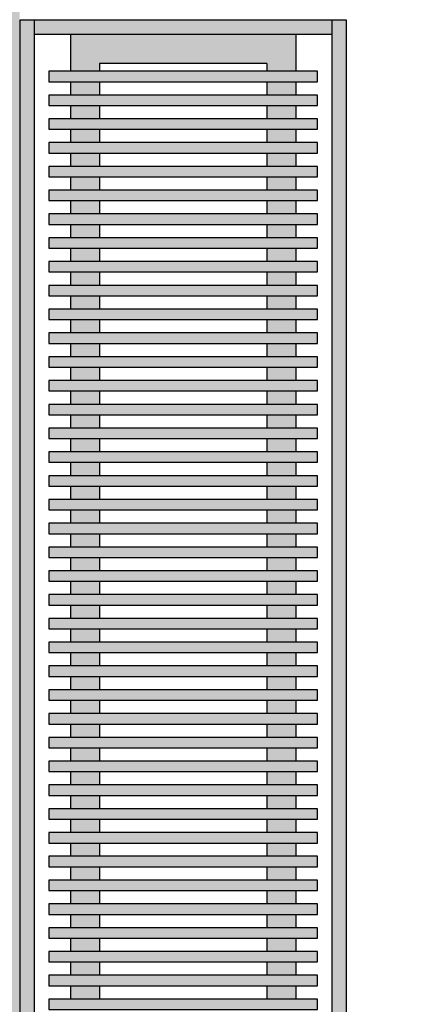
# Model space of a CAD drawing. Units: inches. Extents: x 3592 to 4861, y 1650 to 2243.
# Tile 20 of 30: x 4047 to 4068, y 2072 to 2125. Entities that reach past the tile are written whole.
import ezdxf

# ---------------------------------------------------------------- set-up
doc = ezdxf.new("R2010")
doc.units = ezdxf.units.IN
doc.layers.add('A-FURN', color=9, linetype='Continuous', lineweight=13)
doc.layers.add('estofado', color=7, linetype='Continuous', lineweight=25)
doc.layers.add('A-WALL-PATT', color=252, linetype='Continuous', lineweight=13, true_color=0x939598)
doc.layers.add('MOBIL', color=7, linetype='Continuous')

# ---------------------------------------------------------------- blocks, each defined once
blk = doc.blocks.new('Aparador Aido WV')
at = {"layer": 'MOBIL'}
h = blk.add_hatch(color=256, dxfattribs=at)
h.set_gradient(color1=(226, 228, 228), one_color=1, tint=1, name='CYLINDER')
h.paths.add_polyline_path([(0.9, -0.02), (0.9, 0), (-0.9, 0), (-0.9, -0.02)])
h = blk.add_hatch(color=256, dxfattribs=at)
h.set_gradient(color1=(226, 228, 228), one_color=1, tint=1)
h.paths.add_polyline_path([(-0.88, -0.02), (-0.9, -0.02), (-0.9, -0.43), (-0.88, -0.43)])
h = blk.add_hatch(color=256, dxfattribs=at)
h.set_gradient(color1=(106, 79, 62), color2=(55, 41, 32), one_color=1, tint=0.17)
h.paths.add_polyline_path([(-0.8151, -0.0402), (-0.8295, -0.0402), (-0.8295, -0.4098), (-0.8151, -0.4098)])
h = blk.add_hatch(color=256, dxfattribs=at)
h.set_gradient(color1=(106, 79, 62), color2=(55, 41, 32), one_color=1, tint=0.17)
h.paths.add_polyline_path([(-0.7967, -0.0402), (-0.7967, -0.4098), (-0.7823, -0.4098), (-0.7823, -0.0402)])
h = blk.add_hatch(color=256, dxfattribs=at)
h.set_gradient(color1=(106, 79, 62), color2=(55, 41, 32), one_color=1, tint=0.17)
h.paths.add_polyline_path([(-0.764, -0.0402), (-0.764, -0.4098), (-0.7496, -0.4098), (-0.7496, -0.0402)])
h = blk.add_hatch(color=256, dxfattribs=at)
h.set_gradient(color1=(106, 79, 62), color2=(55, 41, 32), one_color=1, tint=0.17)
h.paths.add_polyline_path([(-0.7312, -0.0402), (-0.7312, -0.4098), (-0.7168, -0.4098), (-0.7168, -0.0402)])
h = blk.add_hatch(color=256, dxfattribs=at)
h.set_gradient(color1=(106, 79, 62), color2=(55, 41, 32), one_color=1, tint=0.17)
h.paths.add_polyline_path([(-0.6985, -0.0402), (-0.6985, -0.4098), (-0.6841, -0.4098), (-0.6841, -0.0402)])
h = blk.add_hatch(color=256, dxfattribs=at)
h.set_gradient(color1=(106, 79, 62), color2=(55, 41, 32), one_color=1, tint=0.17)
h.paths.add_polyline_path([(-0.6657, -0.0402), (-0.6657, -0.4098), (-0.6513, -0.4098), (-0.6513, -0.0402)])
h = blk.add_hatch(color=256, dxfattribs=at)
h.set_gradient(color1=(106, 79, 62), color2=(55, 41, 32), one_color=1, tint=0.17)
h.paths.add_polyline_path([(-0.633, -0.0402), (-0.633, -0.4098), (-0.6186, -0.4098), (-0.6186, -0.0402)])
h = blk.add_hatch(color=256, dxfattribs=at)
h.set_gradient(color1=(106, 79, 62), color2=(55, 41, 32), one_color=1, tint=0.17)
h.paths.add_polyline_path([(-0.6002, -0.0402), (-0.6002, -0.4098), (-0.5858, -0.4098), (-0.5858, -0.0402)])
h = blk.add_hatch(color=256, dxfattribs=at)
h.set_gradient(color1=(106, 79, 62), color2=(55, 41, 32), one_color=1, tint=0.17)
h.paths.add_polyline_path([(-0.5675, -0.4098), (-0.5531, -0.4098), (-0.5531, -0.0402), (-0.5675, -0.0402)])
h = blk.add_hatch(color=256, dxfattribs=at)
h.set_gradient(color1=(106, 79, 62), color2=(55, 41, 32), one_color=1, tint=0.17)
h.paths.add_polyline_path([(-0.5347, -0.0402), (-0.5347, -0.4098), (-0.5203, -0.4098), (-0.5203, -0.0402)])
h = blk.add_hatch(color=256, dxfattribs=at)
h.set_gradient(color1=(106, 79, 62), color2=(55, 41, 32), one_color=1, tint=0.17)
h.paths.add_polyline_path([(-0.5019, -0.0402), (-0.5019, -0.4098), (-0.4876, -0.4098), (-0.4876, -0.0402)])
h = blk.add_hatch(color=256, dxfattribs=at)
h.set_gradient(color1=(106, 79, 62), color2=(55, 41, 32), one_color=1, tint=0.17)
h.paths.add_polyline_path([(-0.4692, -0.0402), (-0.4692, -0.4098), (-0.4548, -0.4098), (-0.4548, -0.0402)])
h = blk.add_hatch(color=256, dxfattribs=at)
h.set_gradient(color1=(106, 79, 62), color2=(55, 41, 32), one_color=1, tint=0.17)
h.paths.add_polyline_path([(-0.4364, -0.0402), (-0.4364, -0.4098), (-0.4221, -0.4098), (-0.4221, -0.0402)])
h = blk.add_hatch(color=256, dxfattribs=at)
h.set_gradient(color1=(106, 79, 62), color2=(55, 41, 32), one_color=1, tint=0.17)
h.paths.add_polyline_path([(-0.4037, -0.0402), (-0.4037, -0.4098), (-0.3893, -0.4098), (-0.3893, -0.0402)])
h = blk.add_hatch(color=256, dxfattribs=at)
h.set_gradient(color1=(106, 79, 62), color2=(55, 41, 32), one_color=1, tint=0.17)
h.paths.add_polyline_path([(-0.3709, -0.0402), (-0.3709, -0.4098), (-0.3566, -0.4098), (-0.3566, -0.0402)])
h = blk.add_hatch(color=256, dxfattribs=at)
h.set_gradient(color1=(106, 79, 62), color2=(55, 41, 32), one_color=1, tint=0.17)
h.paths.add_polyline_path([(-0.3382, -0.0402), (-0.3382, -0.4098), (-0.3238, -0.4098), (-0.3238, -0.0402)])
h = blk.add_hatch(color=256, dxfattribs=at)
h.set_gradient(color1=(106, 79, 62), color2=(55, 41, 32), one_color=1, tint=0.17)
h.paths.add_polyline_path([(-0.3054, -0.0402), (-0.3054, -0.4098), (-0.2911, -0.4098), (-0.2911, -0.0402)])
h = blk.add_hatch(color=256, dxfattribs=at)
h.set_gradient(color1=(106, 79, 62), color2=(55, 41, 32), one_color=1, tint=0.17)
h.paths.add_polyline_path([(-0.2727, -0.0402), (-0.2727, -0.4098), (-0.2583, -0.4098), (-0.2583, -0.0402)])
h = blk.add_hatch(color=256, dxfattribs=at)
h.set_gradient(color1=(106, 79, 62), color2=(55, 41, 32), one_color=1, tint=0.17)
h.paths.add_polyline_path([(-0.2399, -0.0402), (-0.2399, -0.4098), (-0.2256, -0.4098), (-0.2256, -0.0402)])
h = blk.add_hatch(color=256, dxfattribs=at)
h.set_gradient(color1=(106, 79, 62), color2=(55, 41, 32), one_color=1, tint=0.17)
h.paths.add_polyline_path([(-0.2072, -0.4098), (-0.1928, -0.4098), (-0.1928, -0.0402), (-0.2072, -0.0402)])
h = blk.add_hatch(color=256, dxfattribs=at)
h.set_gradient(color1=(106, 79, 62), color2=(55, 41, 32), one_color=1, tint=0.17)
h.paths.add_polyline_path([(-0.1744, -0.0402), (-0.1744, -0.4098), (-0.1601, -0.4098), (-0.1601, -0.0402)])
h = blk.add_hatch(color=256, dxfattribs=at)
h.set_gradient(color1=(106, 79, 62), color2=(55, 41, 32), one_color=1, tint=0.17)
h.paths.add_polyline_path([(-0.1417, -0.0402), (-0.1417, -0.4098), (-0.1273, -0.4098), (-0.1273, -0.0402)])
h = blk.add_hatch(color=256, dxfattribs=at)
h.set_gradient(color1=(106, 79, 62), color2=(55, 41, 32), one_color=1, tint=0.17)
h.paths.add_polyline_path([(-0.1089, -0.0402), (-0.1089, -0.4098), (-0.0946, -0.4098), (-0.0946, -0.0402)])
h = blk.add_hatch(color=256, dxfattribs=at)
h.set_gradient(color1=(106, 79, 62), color2=(55, 41, 32), one_color=1, tint=0.17)
h.paths.add_polyline_path([(-0.0762, -0.0402), (-0.0762, -0.4098), (-0.0618, -0.4098), (-0.0618, -0.0402)])
h = blk.add_hatch(color=256, dxfattribs=at)
h.set_gradient(color1=(106, 79, 62), color2=(55, 41, 32), one_color=1, tint=0.17)
h.paths.add_polyline_path([(-0.0434, -0.0402), (-0.0434, -0.4098), (-0.0291, -0.4098), (-0.0291, -0.0402)])
h = blk.add_hatch(color=256, dxfattribs=at)
h.set_gradient(color1=(106, 79, 62), color2=(55, 41, 32), one_color=1, tint=0.17)
h.paths.add_polyline_path([(-0.0107, -0.0402), (-0.0107, -0.4098), (0.0037, -0.4098), (0.0037, -0.0402)])
h = blk.add_hatch(color=256, dxfattribs=at)
h.set_gradient(color1=(106, 79, 62), color2=(55, 41, 32), one_color=1, tint=0.17)
h.paths.add_polyline_path([(0.0221, -0.0402), (0.0221, -0.4098), (0.0364, -0.4098), (0.0364, -0.0402)])
h = blk.add_hatch(color=256, dxfattribs=at)
h.set_gradient(color1=(106, 79, 62), color2=(55, 41, 32), one_color=1, tint=0.17)
h.paths.add_polyline_path([(0.0548, -0.0402), (0.0548, -0.4098), (0.0692, -0.4098), (0.0692, -0.0402)])
h = blk.add_hatch(color=256, dxfattribs=at)
h.set_gradient(color1=(106, 79, 62), color2=(55, 41, 32), one_color=1, tint=0.17)
h.paths.add_polyline_path([(0.1019, -0.0402), (0.0876, -0.0402), (0.0876, -0.4098), (0.1019, -0.4098)])
h = blk.add_hatch(color=256, dxfattribs=at)
h.set_gradient(color1=(106, 79, 62), color2=(55, 41, 32), one_color=1, tint=0.17)
h.paths.add_polyline_path([(0.1203, -0.0402), (0.1203, -0.4098), (0.1347, -0.4098), (0.1347, -0.0402)])
h = blk.add_hatch(color=256, dxfattribs=at)
h.set_gradient(color1=(106, 79, 62), color2=(55, 41, 32), one_color=1, tint=0.17)
h.paths.add_polyline_path([(0.1531, -0.0402), (0.1531, -0.4098), (0.1675, -0.4098), (0.1675, -0.0402)])
h = blk.add_hatch(color=256, dxfattribs=at)
h.set_gradient(color1=(106, 79, 62), color2=(55, 41, 32), one_color=1, tint=0.17)
h.paths.add_polyline_path([(0.1858, -0.0402), (0.1858, -0.4098), (0.2002, -0.4098), (0.2002, -0.0402)])
h = blk.add_hatch(color=256, dxfattribs=at)
h.set_gradient(color1=(106, 79, 62), color2=(55, 41, 32), one_color=1, tint=0.17)
h.paths.add_polyline_path([(0.2186, -0.0402), (0.2186, -0.4098), (0.233, -0.4098), (0.233, -0.0402)])
h = blk.add_hatch(color=256, dxfattribs=at)
h.set_gradient(color1=(106, 79, 62), color2=(55, 41, 32), one_color=1, tint=0.17)
h.paths.add_polyline_path([(0.2513, -0.0402), (0.2513, -0.4098), (0.2657, -0.4098), (0.2657, -0.0402)])
h = blk.add_hatch(color=256, dxfattribs=at)
h.set_gradient(color1=(106, 79, 62), color2=(55, 41, 32), one_color=1, tint=0.17)
h.paths.add_polyline_path([(0.2841, -0.0402), (0.2841, -0.4098), (0.2985, -0.4098), (0.2985, -0.0402)])
h = blk.add_hatch(color=256, dxfattribs=at)
h.set_gradient(color1=(106, 79, 62), color2=(55, 41, 32), one_color=1, tint=0.17)
h.paths.add_polyline_path([(0.3168, -0.0402), (0.3168, -0.4098), (0.3312, -0.4098), (0.3312, -0.0402)])
h = blk.add_hatch(color=256, dxfattribs=at)
h.set_gradient(color1=(106, 79, 62), color2=(55, 41, 32), one_color=1, tint=0.17)
h.paths.add_polyline_path([(0.3496, -0.0402), (0.3496, -0.4098), (0.364, -0.4098), (0.364, -0.0402)])
h = blk.add_hatch(color=256, dxfattribs=at)
h.set_gradient(color1=(106, 79, 62), color2=(55, 41, 32), one_color=1, tint=0.17)
h.paths.add_polyline_path([(0.3823, -0.0402), (0.3823, -0.4098), (0.3967, -0.4098), (0.3967, -0.0402)])
h = blk.add_hatch(color=256, dxfattribs=at)
h.set_gradient(color1=(106, 79, 62), color2=(55, 41, 32), one_color=1, tint=0.17)
h.paths.add_polyline_path([(0.4151, -0.4098), (0.4295, -0.4098), (0.4295, -0.0402), (0.4151, -0.0402)])
h = blk.add_hatch(color=256, dxfattribs=at)
h.set_gradient(color1=(106, 79, 62), color2=(55, 41, 32), one_color=1, tint=0.17)
h.paths.add_polyline_path([(0.4479, -0.0402), (0.4479, -0.4098), (0.4622, -0.4098), (0.4622, -0.0402)])
h = blk.add_hatch(color=256, dxfattribs=at)
h.set_gradient(color1=(106, 79, 62), color2=(157, 117, 92), one_color=1, tint=0.49)
h.paths.add_polyline_path([(-0.84, -0.11), (-0.8295, -0.11), (-0.8295, -0.07), (-0.88, -0.07), (-0.88, -0.38), (-0.8295, -0.38), (-0.8295, -0.34), (-0.84, -0.34)])
h = blk.add_hatch(color=256, dxfattribs=at)
h.set_gradient(color1=(106, 79, 62), color2=(157, 117, 92), one_color=1, tint=0.49)
h.paths.add_polyline_path([(-0.7967, -0.07), (-0.8151, -0.07), (-0.8151, -0.11), (-0.7967, -0.11)])
h = blk.add_hatch(color=256, dxfattribs=at)
h.set_gradient(color1=(106, 79, 62), color2=(157, 117, 92), one_color=1, tint=0.49)
h.paths.add_polyline_path([(-0.764, -0.07), (-0.7823, -0.07), (-0.7823, -0.11), (-0.764, -0.11)])
h = blk.add_hatch(color=256, dxfattribs=at)
h.set_gradient(color1=(106, 79, 62), color2=(157, 117, 92), one_color=1, tint=0.49)
h.paths.add_polyline_path([(-0.7312, -0.07), (-0.7496, -0.07), (-0.7496, -0.11), (-0.7312, -0.11)])
h = blk.add_hatch(color=256, dxfattribs=at)
h.set_gradient(color1=(106, 79, 62), color2=(157, 117, 92), one_color=1, tint=0.49)
h.paths.add_polyline_path([(-0.6985, -0.07), (-0.7168, -0.07), (-0.7168, -0.11), (-0.6985, -0.11)])
h = blk.add_hatch(color=256, dxfattribs=at)
h.set_gradient(color1=(106, 79, 62), color2=(157, 117, 92), one_color=1, tint=0.49)
h.paths.add_polyline_path([(-0.6657, -0.07), (-0.6841, -0.07), (-0.6841, -0.11), (-0.6657, -0.11)])
h = blk.add_hatch(color=256, dxfattribs=at)
h.set_gradient(color1=(106, 79, 62), color2=(157, 117, 92), one_color=1, tint=0.49)
h.paths.add_polyline_path([(-0.633, -0.07), (-0.6513, -0.07), (-0.6513, -0.11), (-0.633, -0.11)])
h = blk.add_hatch(color=256, dxfattribs=at)
h.set_gradient(color1=(106, 79, 62), color2=(157, 117, 92), one_color=1, tint=0.49)
h.paths.add_polyline_path([(-0.6002, -0.07), (-0.6186, -0.07), (-0.6186, -0.11), (-0.6002, -0.11)])
h = blk.add_hatch(color=256, dxfattribs=at)
h.set_gradient(color1=(106, 79, 62), color2=(157, 117, 92), one_color=1, tint=0.49)
h.paths.add_polyline_path([(-0.5675, -0.07), (-0.5858, -0.07), (-0.5858, -0.11), (-0.5675, -0.11)])
h = blk.add_hatch(color=256, dxfattribs=at)
h.set_gradient(color1=(106, 79, 62), color2=(157, 117, 92), one_color=1, tint=0.49)
h.paths.add_polyline_path([(-0.5347, -0.07), (-0.5531, -0.07), (-0.5531, -0.11), (-0.5347, -0.11)])
h = blk.add_hatch(color=256, dxfattribs=at)
h.set_gradient(color1=(106, 79, 62), color2=(157, 117, 92), one_color=1, tint=0.49)
h.paths.add_polyline_path([(-0.5019, -0.07), (-0.5203, -0.07), (-0.5203, -0.11), (-0.5019, -0.11)])
h = blk.add_hatch(color=256, dxfattribs=at)
h.set_gradient(color1=(106, 79, 62), color2=(157, 117, 92), one_color=1, tint=0.49)
h.paths.add_polyline_path([(-0.4692, -0.07), (-0.4876, -0.07), (-0.4876, -0.11), (-0.4692, -0.11)])
h = blk.add_hatch(color=256, dxfattribs=at)
h.set_gradient(color1=(106, 79, 62), color2=(157, 117, 92), one_color=1, tint=0.49)
h.paths.add_polyline_path([(-0.4364, -0.07), (-0.4548, -0.07), (-0.4548, -0.11), (-0.4364, -0.11)])
h = blk.add_hatch(color=256, dxfattribs=at)
h.set_gradient(color1=(106, 79, 62), color2=(157, 117, 92), one_color=1, tint=0.49)
h.paths.add_polyline_path([(-0.4037, -0.07), (-0.4221, -0.07), (-0.4221, -0.11), (-0.4037, -0.11)])
h = blk.add_hatch(color=256, dxfattribs=at)
h.set_gradient(color1=(106, 79, 62), color2=(157, 117, 92), one_color=1, tint=0.49)
h.paths.add_polyline_path([(-0.3709, -0.07), (-0.3893, -0.07), (-0.3893, -0.11), (-0.3709, -0.11)])
h = blk.add_hatch(color=256, dxfattribs=at)
h.set_gradient(color1=(106, 79, 62), color2=(157, 117, 92), one_color=1, tint=0.49)
h.paths.add_polyline_path([(-0.3382, -0.07), (-0.3566, -0.07), (-0.3566, -0.11), (-0.3382, -0.11)])
h = blk.add_hatch(color=256, dxfattribs=at)
h.set_gradient(color1=(106, 79, 62), color2=(157, 117, 92), one_color=1, tint=0.49)
h.paths.add_polyline_path([(-0.3054, -0.07), (-0.3238, -0.07), (-0.3238, -0.11), (-0.3054, -0.11)])
h = blk.add_hatch(color=256, dxfattribs=at)
h.set_gradient(color1=(106, 79, 62), color2=(157, 117, 92), one_color=1, tint=0.49)
h.paths.add_polyline_path([(-0.2727, -0.07), (-0.2911, -0.07), (-0.2911, -0.11), (-0.2727, -0.11)])
h = blk.add_hatch(color=256, dxfattribs=at)
h.set_gradient(color1=(106, 79, 62), color2=(157, 117, 92), one_color=1, tint=0.49)
h.paths.add_polyline_path([(-0.2399, -0.07), (-0.2583, -0.07), (-0.2583, -0.11), (-0.2399, -0.11)])
h = blk.add_hatch(color=256, dxfattribs=at)
h.set_gradient(color1=(106, 79, 62), color2=(157, 117, 92), one_color=1, tint=0.49)
h.paths.add_polyline_path([(-0.2072, -0.07), (-0.2256, -0.07), (-0.2256, -0.11), (-0.2072, -0.11)])
h = blk.add_hatch(color=256, dxfattribs=at)
h.set_gradient(color1=(106, 79, 62), color2=(157, 117, 92), one_color=1, tint=0.49)
h.paths.add_polyline_path([(-0.1744, -0.07), (-0.1928, -0.07), (-0.1928, -0.11), (-0.1744, -0.11)])
h = blk.add_hatch(color=256, dxfattribs=at)
h.set_gradient(color1=(106, 79, 62), color2=(157, 117, 92), one_color=1, tint=0.49)
h.paths.add_polyline_path([(-0.1417, -0.07), (-0.1601, -0.07), (-0.1601, -0.11), (-0.1417, -0.11)])
h = blk.add_hatch(color=256, dxfattribs=at)
h.set_gradient(color1=(106, 79, 62), color2=(157, 117, 92), one_color=1, tint=0.49)
h.paths.add_polyline_path([(-0.1089, -0.07), (-0.1273, -0.07), (-0.1273, -0.11), (-0.1089, -0.11)])
h = blk.add_hatch(color=256, dxfattribs=at)
h.set_gradient(color1=(106, 79, 62), color2=(157, 117, 92), one_color=1, tint=0.49)
h.paths.add_polyline_path([(-0.0762, -0.07), (-0.0946, -0.07), (-0.0946, -0.11), (-0.0762, -0.11)])
h = blk.add_hatch(color=256, dxfattribs=at)
h.set_gradient(color1=(106, 79, 62), color2=(157, 117, 92), one_color=1, tint=0.49)
h.paths.add_polyline_path([(-0.0434, -0.07), (-0.0618, -0.07), (-0.0618, -0.11), (-0.0434, -0.11)])
h = blk.add_hatch(color=256, dxfattribs=at)
h.set_gradient(color1=(106, 79, 62), color2=(157, 117, 92), one_color=1, tint=0.49)
h.paths.add_polyline_path([(-0.0107, -0.07), (-0.0291, -0.07), (-0.0291, -0.11), (-0.0107, -0.11)])
h = blk.add_hatch(color=256, dxfattribs=at)
h.set_gradient(color1=(106, 79, 62), color2=(157, 117, 92), one_color=1, tint=0.49)
h.paths.add_polyline_path([(0.0221, -0.07), (0.0037, -0.07), (0.0037, -0.11), (0.0221, -0.11)])
h = blk.add_hatch(color=256, dxfattribs=at)
h.set_gradient(color1=(106, 79, 62), color2=(157, 117, 92), one_color=1, tint=0.49)
h.paths.add_polyline_path([(0.0548, -0.07), (0.0364, -0.07), (0.0364, -0.11), (0.0548, -0.11)])
h = blk.add_hatch(color=256, dxfattribs=at)
h.set_gradient(color1=(106, 79, 62), color2=(157, 117, 92), one_color=1, tint=0.49)
h.paths.add_polyline_path([(0.0876, -0.07), (0.0692, -0.07), (0.0692, -0.11), (0.0876, -0.11)])
h = blk.add_hatch(color=256, dxfattribs=at)
h.set_gradient(color1=(106, 79, 62), color2=(157, 117, 92), one_color=1, tint=0.49)
h.paths.add_polyline_path([(0.1203, -0.07), (0.1019, -0.07), (0.1019, -0.11), (0.1203, -0.11)])
h = blk.add_hatch(color=256, dxfattribs=at)
h.set_gradient(color1=(106, 79, 62), color2=(157, 117, 92), one_color=1, tint=0.49)
h.paths.add_polyline_path([(0.1531, -0.07), (0.1347, -0.07), (0.1347, -0.11), (0.1531, -0.11)])
h = blk.add_hatch(color=256, dxfattribs=at)
h.set_gradient(color1=(106, 79, 62), color2=(157, 117, 92), one_color=1, tint=0.49)
h.paths.add_polyline_path([(0.1858, -0.07), (0.1675, -0.07), (0.1675, -0.11), (0.1858, -0.11)])
h = blk.add_hatch(color=256, dxfattribs=at)
h.set_gradient(color1=(106, 79, 62), color2=(157, 117, 92), one_color=1, tint=0.49)
h.paths.add_polyline_path([(0.2186, -0.07), (0.2002, -0.07), (0.2002, -0.11), (0.2186, -0.11)])
h = blk.add_hatch(color=256, dxfattribs=at)
h.set_gradient(color1=(106, 79, 62), color2=(157, 117, 92), one_color=1, tint=0.49)
h.paths.add_polyline_path([(0.2513, -0.07), (0.233, -0.07), (0.233, -0.11), (0.2513, -0.11)])
h = blk.add_hatch(color=256, dxfattribs=at)
h.set_gradient(color1=(106, 79, 62), color2=(157, 117, 92), one_color=1, tint=0.49)
h.paths.add_polyline_path([(0.2841, -0.07), (0.2657, -0.07), (0.2657, -0.11), (0.2841, -0.11)])
h = blk.add_hatch(color=256, dxfattribs=at)
h.set_gradient(color1=(106, 79, 62), color2=(157, 117, 92), one_color=1, tint=0.49)
h.paths.add_polyline_path([(0.3168, -0.07), (0.2985, -0.07), (0.2985, -0.11), (0.3168, -0.11)])
h = blk.add_hatch(color=256, dxfattribs=at)
h.set_gradient(color1=(106, 79, 62), color2=(157, 117, 92), one_color=1, tint=0.49)
h.paths.add_polyline_path([(0.3496, -0.07), (0.3312, -0.07), (0.3312, -0.11), (0.3496, -0.11)])
h = blk.add_hatch(color=256, dxfattribs=at)
h.set_gradient(color1=(106, 79, 62), color2=(157, 117, 92), one_color=1, tint=0.49)
h.paths.add_polyline_path([(0.3823, -0.07), (0.364, -0.07), (0.364, -0.11), (0.3823, -0.11)])
h = blk.add_hatch(color=256, dxfattribs=at)
h.set_gradient(color1=(106, 79, 62), color2=(157, 117, 92), one_color=1, tint=0.49)
h.paths.add_polyline_path([(0.4151, -0.07), (0.3967, -0.07), (0.3967, -0.11), (0.4151, -0.11)])
h = blk.add_hatch(color=256, dxfattribs=at)
h.set_gradient(color1=(106, 79, 62), color2=(157, 117, 92), one_color=1, tint=0.49)
h.paths.add_polyline_path([(0.4479, -0.07), (0.4295, -0.07), (0.4295, -0.11), (0.4479, -0.11)])
h = blk.add_hatch(color=256, dxfattribs=at)
h.set_gradient(color1=(106, 79, 62), color2=(157, 117, 92), one_color=1, tint=0.49)
h.paths.add_polyline_path([(-0.7967, -0.34), (-0.8151, -0.34), (-0.8151, -0.38), (-0.7967, -0.38)])
h = blk.add_hatch(color=256, dxfattribs=at)
h.set_gradient(color1=(106, 79, 62), color2=(157, 117, 92), one_color=1, tint=0.49)
h.paths.add_polyline_path([(-0.764, -0.34), (-0.7823, -0.34), (-0.7823, -0.38), (-0.764, -0.38)])
h = blk.add_hatch(color=256, dxfattribs=at)
h.set_gradient(color1=(106, 79, 62), color2=(157, 117, 92), one_color=1, tint=0.49)
h.paths.add_polyline_path([(-0.7312, -0.34), (-0.7496, -0.34), (-0.7496, -0.38), (-0.7312, -0.38)])
h = blk.add_hatch(color=256, dxfattribs=at)
h.set_gradient(color1=(106, 79, 62), color2=(157, 117, 92), one_color=1, tint=0.49)
h.paths.add_polyline_path([(-0.6985, -0.34), (-0.7168, -0.34), (-0.7168, -0.38), (-0.6985, -0.38)])
h = blk.add_hatch(color=256, dxfattribs=at)
h.set_gradient(color1=(106, 79, 62), color2=(157, 117, 92), one_color=1, tint=0.49)
h.paths.add_polyline_path([(-0.6657, -0.34), (-0.6841, -0.34), (-0.6841, -0.38), (-0.6657, -0.38)])
h = blk.add_hatch(color=256, dxfattribs=at)
h.set_gradient(color1=(106, 79, 62), color2=(157, 117, 92), one_color=1, tint=0.49)
h.paths.add_polyline_path([(-0.633, -0.34), (-0.6513, -0.34), (-0.6513, -0.38), (-0.633, -0.38)])
h = blk.add_hatch(color=256, dxfattribs=at)
h.set_gradient(color1=(106, 79, 62), color2=(157, 117, 92), one_color=1, tint=0.49)
h.paths.add_polyline_path([(-0.6002, -0.34), (-0.6186, -0.34), (-0.6186, -0.38), (-0.6002, -0.38)])
h = blk.add_hatch(color=256, dxfattribs=at)
h.set_gradient(color1=(106, 79, 62), color2=(157, 117, 92), one_color=1, tint=0.49)
h.paths.add_polyline_path([(-0.5675, -0.34), (-0.5858, -0.34), (-0.5858, -0.38), (-0.5675, -0.38)])
h = blk.add_hatch(color=256, dxfattribs=at)
h.set_gradient(color1=(106, 79, 62), color2=(157, 117, 92), one_color=1, tint=0.49)
h.paths.add_polyline_path([(-0.5347, -0.34), (-0.5531, -0.34), (-0.5531, -0.38), (-0.5347, -0.38)])
h = blk.add_hatch(color=256, dxfattribs=at)
h.set_gradient(color1=(106, 79, 62), color2=(157, 117, 92), one_color=1, tint=0.49)
h.paths.add_polyline_path([(-0.5019, -0.34), (-0.5203, -0.34), (-0.5203, -0.38), (-0.5019, -0.38)])
h = blk.add_hatch(color=256, dxfattribs=at)
h.set_gradient(color1=(106, 79, 62), color2=(157, 117, 92), one_color=1, tint=0.49)
h.paths.add_polyline_path([(-0.4692, -0.34), (-0.4876, -0.34), (-0.4876, -0.38), (-0.4692, -0.38)])
h = blk.add_hatch(color=256, dxfattribs=at)
h.set_gradient(color1=(106, 79, 62), color2=(157, 117, 92), one_color=1, tint=0.49)
h.paths.add_polyline_path([(-0.4364, -0.34), (-0.4548, -0.34), (-0.4548, -0.38), (-0.4364, -0.38)])
h = blk.add_hatch(color=256, dxfattribs=at)
h.set_gradient(color1=(106, 79, 62), color2=(157, 117, 92), one_color=1, tint=0.49)
h.paths.add_polyline_path([(-0.4037, -0.34), (-0.4221, -0.34), (-0.4221, -0.38), (-0.4037, -0.38)])
h = blk.add_hatch(color=256, dxfattribs=at)
h.set_gradient(color1=(106, 79, 62), color2=(157, 117, 92), one_color=1, tint=0.49)
h.paths.add_polyline_path([(-0.3709, -0.34), (-0.3893, -0.34), (-0.3893, -0.38), (-0.3709, -0.38)])
h = blk.add_hatch(color=256, dxfattribs=at)
h.set_gradient(color1=(106, 79, 62), color2=(157, 117, 92), one_color=1, tint=0.49)
h.paths.add_polyline_path([(-0.3382, -0.34), (-0.3566, -0.34), (-0.3566, -0.38), (-0.3382, -0.38)])
h = blk.add_hatch(color=256, dxfattribs=at)
h.set_gradient(color1=(106, 79, 62), color2=(157, 117, 92), one_color=1, tint=0.49)
h.paths.add_polyline_path([(-0.3054, -0.34), (-0.3238, -0.34), (-0.3238, -0.38), (-0.3054, -0.38)])
h = blk.add_hatch(color=256, dxfattribs=at)
h.set_gradient(color1=(106, 79, 62), color2=(157, 117, 92), one_color=1, tint=0.49)
h.paths.add_polyline_path([(-0.2727, -0.34), (-0.2911, -0.34), (-0.2911, -0.38), (-0.2727, -0.38)])
h = blk.add_hatch(color=256, dxfattribs=at)
h.set_gradient(color1=(106, 79, 62), color2=(157, 117, 92), one_color=1, tint=0.49)
h.paths.add_polyline_path([(-0.2399, -0.34), (-0.2583, -0.34), (-0.2583, -0.38), (-0.2399, -0.38)])
h = blk.add_hatch(color=256, dxfattribs=at)
h.set_gradient(color1=(106, 79, 62), color2=(157, 117, 92), one_color=1, tint=0.49)
h.paths.add_polyline_path([(-0.2072, -0.34), (-0.2256, -0.34), (-0.2256, -0.38), (-0.2072, -0.38)])
h = blk.add_hatch(color=256, dxfattribs=at)
h.set_gradient(color1=(106, 79, 62), color2=(157, 117, 92), one_color=1, tint=0.49)
h.paths.add_polyline_path([(-0.1744, -0.34), (-0.1928, -0.34), (-0.1928, -0.38), (-0.1744, -0.38)])
h = blk.add_hatch(color=256, dxfattribs=at)
h.set_gradient(color1=(106, 79, 62), color2=(157, 117, 92), one_color=1, tint=0.49)
h.paths.add_polyline_path([(-0.1417, -0.34), (-0.1601, -0.34), (-0.1601, -0.38), (-0.1417, -0.38)])
h = blk.add_hatch(color=256, dxfattribs=at)
h.set_gradient(color1=(106, 79, 62), color2=(157, 117, 92), one_color=1, tint=0.49)
h.paths.add_polyline_path([(-0.1089, -0.34), (-0.1273, -0.34), (-0.1273, -0.38), (-0.1089, -0.38)])
h = blk.add_hatch(color=256, dxfattribs=at)
h.set_gradient(color1=(106, 79, 62), color2=(157, 117, 92), one_color=1, tint=0.49)
h.paths.add_polyline_path([(-0.0762, -0.34), (-0.0946, -0.34), (-0.0946, -0.38), (-0.0762, -0.38)])
h = blk.add_hatch(color=256, dxfattribs=at)
h.set_gradient(color1=(106, 79, 62), color2=(157, 117, 92), one_color=1, tint=0.49)
h.paths.add_polyline_path([(-0.0434, -0.34), (-0.0618, -0.34), (-0.0618, -0.38), (-0.0434, -0.38)])
h = blk.add_hatch(color=256, dxfattribs=at)
h.set_gradient(color1=(106, 79, 62), color2=(157, 117, 92), one_color=1, tint=0.49)
h.paths.add_polyline_path([(-0.0107, -0.34), (-0.0291, -0.34), (-0.0291, -0.38), (-0.0107, -0.38)])
h = blk.add_hatch(color=256, dxfattribs=at)
h.set_gradient(color1=(106, 79, 62), color2=(157, 117, 92), one_color=1, tint=0.49)
h.paths.add_polyline_path([(0.0221, -0.34), (0.0037, -0.34), (0.0037, -0.38), (0.0221, -0.38)])
h = blk.add_hatch(color=256, dxfattribs=at)
h.set_gradient(color1=(106, 79, 62), color2=(157, 117, 92), one_color=1, tint=0.49)
h.paths.add_polyline_path([(0.0548, -0.34), (0.0364, -0.34), (0.0364, -0.38), (0.0548, -0.38)])
h = blk.add_hatch(color=256, dxfattribs=at)
h.set_gradient(color1=(106, 79, 62), color2=(157, 117, 92), one_color=1, tint=0.49)
h.paths.add_polyline_path([(0.0876, -0.34), (0.0692, -0.34), (0.0692, -0.38), (0.0876, -0.38)])
h = blk.add_hatch(color=256, dxfattribs=at)
h.set_gradient(color1=(106, 79, 62), color2=(157, 117, 92), one_color=1, tint=0.49)
h.paths.add_polyline_path([(0.1203, -0.34), (0.1019, -0.34), (0.1019, -0.38), (0.1203, -0.38)])
h = blk.add_hatch(color=256, dxfattribs=at)
h.set_gradient(color1=(106, 79, 62), color2=(157, 117, 92), one_color=1, tint=0.49)
h.paths.add_polyline_path([(0.1531, -0.34), (0.1347, -0.34), (0.1347, -0.38), (0.1531, -0.38)])
h = blk.add_hatch(color=256, dxfattribs=at)
h.set_gradient(color1=(106, 79, 62), color2=(157, 117, 92), one_color=1, tint=0.49)
h.paths.add_polyline_path([(0.1858, -0.34), (0.1675, -0.34), (0.1675, -0.38), (0.1858, -0.38)])
h = blk.add_hatch(color=256, dxfattribs=at)
h.set_gradient(color1=(106, 79, 62), color2=(157, 117, 92), one_color=1, tint=0.49)
h.paths.add_polyline_path([(0.2186, -0.34), (0.2002, -0.34), (0.2002, -0.38), (0.2186, -0.38)])
h = blk.add_hatch(color=256, dxfattribs=at)
h.set_gradient(color1=(106, 79, 62), color2=(157, 117, 92), one_color=1, tint=0.49)
h.paths.add_polyline_path([(0.2513, -0.34), (0.233, -0.34), (0.233, -0.38), (0.2513, -0.38)])
h = blk.add_hatch(color=256, dxfattribs=at)
h.set_gradient(color1=(106, 79, 62), color2=(157, 117, 92), one_color=1, tint=0.49)
h.paths.add_polyline_path([(0.2841, -0.34), (0.2657, -0.34), (0.2657, -0.38), (0.2841, -0.38)])
h = blk.add_hatch(color=256, dxfattribs=at)
h.set_gradient(color1=(106, 79, 62), color2=(157, 117, 92), one_color=1, tint=0.49)
h.paths.add_polyline_path([(0.3168, -0.34), (0.2985, -0.34), (0.2985, -0.38), (0.3168, -0.38)])
h = blk.add_hatch(color=256, dxfattribs=at)
h.set_gradient(color1=(106, 79, 62), color2=(157, 117, 92), one_color=1, tint=0.49)
h.paths.add_polyline_path([(0.3496, -0.34), (0.3312, -0.34), (0.3312, -0.38), (0.3496, -0.38)])
h = blk.add_hatch(color=256, dxfattribs=at)
h.set_gradient(color1=(106, 79, 62), color2=(157, 117, 92), one_color=1, tint=0.49)
h.paths.add_polyline_path([(0.3823, -0.34), (0.364, -0.34), (0.364, -0.38), (0.3823, -0.38)])
h = blk.add_hatch(color=256, dxfattribs=at)
h.set_gradient(color1=(106, 79, 62), color2=(157, 117, 92), one_color=1, tint=0.49)
h.paths.add_polyline_path([(0.4151, -0.34), (0.3967, -0.34), (0.3967, -0.38), (0.4151, -0.38)])
h = blk.add_hatch(color=256, dxfattribs=at)
h.set_gradient(color1=(106, 79, 62), color2=(157, 117, 92), one_color=1, tint=0.49)
h.paths.add_polyline_path([(0.4479, -0.34), (0.4295, -0.34), (0.4295, -0.38), (0.4479, -0.38)])
h = blk.add_hatch(color=256, dxfattribs=at)
h.set_gradient(color1=(226, 228, 228), one_color=1, tint=1, name='CYLINDER')
h.paths.add_polyline_path([(0.9, -0.45), (0.9, -0.43), (-0.9, -0.43), (-0.9, -0.45)])
at = {"layer": 'estofado', "ltscale": 0.5}
for p, q in [((-0.88, -0.07), (-0.8295, -0.07)), ((-0.8151, -0.07), (-0.7967, -0.07)), ((-0.7823, -0.07), (-0.764, -0.07)), ((-0.7496, -0.07), (-0.7312, -0.07)), ((-0.7168, -0.07), (-0.6985, -0.07)), ((-0.6841, -0.07), (-0.6657, -0.07)), ((-0.6513, -0.07), (-0.633, -0.07)), ((-0.6186, -0.07), (-0.6002, -0.07)), ((-0.5858, -0.07), (-0.5675, -0.07)), ((-0.5531, -0.07), (-0.5347, -0.07)), ((-0.5203, -0.07), (-0.5019, -0.07)), ((-0.4876, -0.07), (-0.4692, -0.07)), ((-0.4548, -0.07), (-0.4364, -0.07)), ((-0.4221, -0.07), (-0.4037, -0.07)), ((-0.3893, -0.07), (-0.3709, -0.07)), ((-0.3566, -0.07), (-0.3382, -0.07)), ((-0.3238, -0.07), (-0.3054, -0.07)), ((-0.2911, -0.07), (-0.2727, -0.07)), ((-0.2583, -0.07), (-0.2399, -0.07)), ((-0.2256, -0.07), (-0.2072, -0.07)), ((-0.1928, -0.07), (-0.1744, -0.07)), ((-0.1601, -0.07), (-0.1417, -0.07)), ((-0.1273, -0.07), (-0.1089, -0.07)), ((-0.0946, -0.07), (-0.0762, -0.07)), ((-0.0618, -0.07), (-0.0434, -0.07)), ((-0.0291, -0.07), (-0.0107, -0.07)), ((0.0037, -0.07), (0.0221, -0.07)), ((0.0364, -0.07), (0.0548, -0.07)), ((0.0692, -0.07), (0.0876, -0.07)), ((0.1019, -0.07), (0.1203, -0.07)), ((0.1347, -0.07), (0.1531, -0.07)), ((0.1675, -0.07), (0.1858, -0.07)), ((0.2002, -0.07), (0.2186, -0.07)), ((0.233, -0.07), (0.2513, -0.07)), ((0.2657, -0.07), (0.2841, -0.07)), ((0.2985, -0.07), (0.3168, -0.07)), ((0.3312, -0.07), (0.3496, -0.07)), ((0.364, -0.07), (0.3823, -0.07)), ((0.3967, -0.07), (0.4151, -0.07)), ((0.4295, -0.07), (0.4479, -0.07)), ((-0.84, -0.11), (-0.84, -0.34)), ((-0.84, -0.11), (-0.8295, -0.11)), ((-0.8151, -0.11), (-0.7967, -0.11)), ((-0.7823, -0.11), (-0.764, -0.11)), ((-0.7496, -0.11), (-0.7312, -0.11)), ((-0.7168, -0.11), (-0.6985, -0.11)), ((-0.6841, -0.11), (-0.6657, -0.11)), ((-0.6513, -0.11), (-0.633, -0.11)), ((-0.6186, -0.11), (-0.6002, -0.11)), ((-0.5858, -0.11), (-0.5675, -0.11)), ((-0.5531, -0.11), (-0.5347, -0.11)), ((-0.5203, -0.11), (-0.5019, -0.11)), ((-0.4876, -0.11), (-0.4692, -0.11)), ((-0.4548, -0.11), (-0.4364, -0.11)), ((-0.4221, -0.11), (-0.4037, -0.11)), ((-0.3893, -0.11), (-0.3709, -0.11)), ((-0.3566, -0.11), (-0.3382, -0.11)), ((-0.3238, -0.11), (-0.3054, -0.11)), ((-0.2911, -0.11), (-0.2727, -0.11)), ((-0.2583, -0.11), (-0.2399, -0.11)), ((-0.2256, -0.11), (-0.2072, -0.11)), ((-0.1928, -0.11), (-0.1744, -0.11)), ((-0.1601, -0.11), (-0.1417, -0.11)), ((-0.1273, -0.11), (-0.1089, -0.11)), ((-0.0946, -0.11), (-0.0762, -0.11)), ((-0.0618, -0.11), (-0.0434, -0.11)), ((-0.0291, -0.11), (-0.0107, -0.11)), ((0.0037, -0.11), (0.0221, -0.11)), ((0.0364, -0.11), (0.0548, -0.11)), ((0.0692, -0.11), (0.0876, -0.11)), ((0.1019, -0.11), (0.1203, -0.11)), ((0.1347, -0.11), (0.1531, -0.11)), ((0.1675, -0.11), (0.1858, -0.11)), ((0.2002, -0.11), (0.2186, -0.11)), ((0.233, -0.11), (0.2513, -0.11)), ((0.2657, -0.11), (0.2841, -0.11)), ((0.2985, -0.11), (0.3168, -0.11)), ((0.3312, -0.11), (0.3496, -0.11)), ((0.364, -0.11), (0.3823, -0.11)), ((0.3967, -0.11), (0.4151, -0.11)), ((0.4295, -0.11), (0.4479, -0.11)), ((-0.84, -0.34), (-0.8295, -0.34)), ((-0.8151, -0.34), (-0.7967, -0.34)), ((-0.7823, -0.34), (-0.764, -0.34)), ((-0.7496, -0.34), (-0.7312, -0.34)), ((-0.7168, -0.34), (-0.6985, -0.34)), ((-0.6841, -0.34), (-0.6657, -0.34)), ((-0.6513, -0.34), (-0.633, -0.34)), ((-0.6186, -0.34), (-0.6002, -0.34)), ((-0.5858, -0.34), (-0.5675, -0.34)), ((-0.5531, -0.34), (-0.5347, -0.34)), ((-0.5203, -0.34), (-0.5019, -0.34)), ((-0.4876, -0.34), (-0.4692, -0.34)), ((-0.4548, -0.34), (-0.4364, -0.34)), ((-0.4221, -0.34), (-0.4037, -0.34)), ((-0.3893, -0.34), (-0.3709, -0.34)), ((-0.3566, -0.34), (-0.3382, -0.34)), ((-0.3238, -0.34), (-0.3054, -0.34)), ((-0.2911, -0.34), (-0.2727, -0.34)), ((-0.2583, -0.34), (-0.2399, -0.34)), ((-0.2256, -0.34), (-0.2072, -0.34)), ((-0.1928, -0.34), (-0.1744, -0.34)), ((-0.1601, -0.34), (-0.1417, -0.34)), ((-0.1273, -0.34), (-0.1089, -0.34)), ((-0.0946, -0.34), (-0.0762, -0.34)), ((-0.0618, -0.34), (-0.0434, -0.34)), ((-0.0291, -0.34), (-0.0107, -0.34)), ((0.0037, -0.34), (0.0221, -0.34)), ((0.0364, -0.34), (0.0548, -0.34)), ((0.0692, -0.34), (0.0876, -0.34)), ((0.1019, -0.34), (0.1203, -0.34)), ((0.1347, -0.34), (0.1531, -0.34)), ((0.1675, -0.34), (0.1858, -0.34)), ((0.2002, -0.34), (0.2186, -0.34)), ((0.233, -0.34), (0.2513, -0.34)), ((0.2657, -0.34), (0.2841, -0.34)), ((0.2985, -0.34), (0.3168, -0.34)), ((0.3312, -0.34), (0.3496, -0.34)), ((0.364, -0.34), (0.3823, -0.34)), ((0.3967, -0.34), (0.4151, -0.34)), ((0.4295, -0.34), (0.4479, -0.34)), ((-0.88, -0.38), (-0.8295, -0.38)), ((-0.84, -0.38), (-0.8295, -0.38)), ((-0.8151, -0.38), (-0.7967, -0.38)), ((-0.7823, -0.38), (-0.764, -0.38)), ((-0.7496, -0.38), (-0.7312, -0.38)), ((-0.7168, -0.38), (-0.6985, -0.38)), ((-0.6841, -0.38), (-0.6657, -0.38)), ((-0.6513, -0.38), (-0.633, -0.38)), ((-0.6186, -0.38), (-0.6002, -0.38)), ((-0.5858, -0.38), (-0.5675, -0.38)), ((-0.5531, -0.38), (-0.5347, -0.38)), ((-0.5203, -0.38), (-0.5019, -0.38)), ((-0.4876, -0.38), (-0.4692, -0.38)), ((-0.4548, -0.38), (-0.4364, -0.38)), ((-0.4221, -0.38), (-0.4037, -0.38)), ((-0.3893, -0.38), (-0.3709, -0.38)), ((-0.3566, -0.38), (-0.3382, -0.38)), ((-0.3238, -0.38), (-0.3054, -0.38)), ((-0.2911, -0.38), (-0.2727, -0.38)), ((-0.2583, -0.38), (-0.2399, -0.38)), ((-0.2256, -0.38), (-0.2072, -0.38)), ((-0.1928, -0.38), (-0.1744, -0.38)), ((-0.1601, -0.38), (-0.1417, -0.38)), ((-0.1273, -0.38), (-0.1089, -0.38)), ((-0.0946, -0.38), (-0.0762, -0.38)), ((-0.0618, -0.38), (-0.0434, -0.38)), ((-0.0291, -0.38), (-0.0107, -0.38)), ((0.0037, -0.38), (0.0221, -0.38)), ((0.0364, -0.38), (0.0548, -0.38)), ((0.0692, -0.38), (0.0876, -0.38)), ((0.1019, -0.38), (0.1203, -0.38)), ((0.1347, -0.38), (0.1531, -0.38)), ((0.1675, -0.38), (0.1858, -0.38)), ((0.2002, -0.38), (0.2186, -0.38)), ((0.233, -0.38), (0.2513, -0.38)), ((0.2657, -0.38), (0.2841, -0.38)), ((0.2985, -0.38), (0.3168, -0.38)), ((0.3312, -0.38), (0.3496, -0.38)), ((0.364, -0.38), (0.3823, -0.38)), ((0.3967, -0.38), (0.4151, -0.38)), ((0.4295, -0.38), (0.4479, -0.38))]:
    blk.add_line(p, q, dxfattribs=at)
for points in [[(-0.8295, -0.0402), (-0.8295, -0.4098), (-0.8151, -0.4098), (-0.8151, -0.0402)], [(-0.7967, -0.0402), (-0.7967, -0.4098), (-0.7823, -0.4098), (-0.7823, -0.0402)], [(-0.764, -0.0402), (-0.764, -0.4098), (-0.7496, -0.4098), (-0.7496, -0.0402)], [(-0.7312, -0.0402), (-0.7312, -0.4098), (-0.7168, -0.4098), (-0.7168, -0.0402)], [(-0.6985, -0.0402), (-0.6985, -0.4098), (-0.6841, -0.4098), (-0.6841, -0.0402)], [(-0.6657, -0.0402), (-0.6657, -0.4098), (-0.6513, -0.4098), (-0.6513, -0.0402)], [(-0.633, -0.0402), (-0.633, -0.4098), (-0.6186, -0.4098), (-0.6186, -0.0402)], [(-0.6002, -0.0402), (-0.6002, -0.4098), (-0.5858, -0.4098), (-0.5858, -0.0402)], [(-0.5675, -0.0402), (-0.5675, -0.4098), (-0.5531, -0.4098), (-0.5531, -0.0402)], [(-0.5347, -0.0402), (-0.5347, -0.4098), (-0.5203, -0.4098), (-0.5203, -0.0402)], [(-0.5019, -0.0402), (-0.5019, -0.4098), (-0.4876, -0.4098), (-0.4876, -0.0402)], [(-0.4692, -0.0402), (-0.4692, -0.4098), (-0.4548, -0.4098), (-0.4548, -0.0402)], [(-0.4364, -0.0402), (-0.4364, -0.4098), (-0.4221, -0.4098), (-0.4221, -0.0402)], [(-0.4037, -0.0402), (-0.4037, -0.4098), (-0.3893, -0.4098), (-0.3893, -0.0402)], [(-0.3709, -0.0402), (-0.3709, -0.4098), (-0.3566, -0.4098), (-0.3566, -0.0402)], [(-0.3382, -0.0402), (-0.3382, -0.4098), (-0.3238, -0.4098), (-0.3238, -0.0402)], [(-0.3054, -0.0402), (-0.3054, -0.4098), (-0.2911, -0.4098), (-0.2911, -0.0402)], [(-0.2727, -0.0402), (-0.2727, -0.4098), (-0.2583, -0.4098), (-0.2583, -0.0402)], [(-0.2399, -0.0402), (-0.2399, -0.4098), (-0.2256, -0.4098), (-0.2256, -0.0402)], [(-0.2072, -0.0402), (-0.2072, -0.4098), (-0.1928, -0.4098), (-0.1928, -0.0402)], [(-0.1744, -0.0402), (-0.1744, -0.4098), (-0.1601, -0.4098), (-0.1601, -0.0402)], [(-0.1417, -0.0402), (-0.1417, -0.4098), (-0.1273, -0.4098), (-0.1273, -0.0402)], [(-0.1089, -0.0402), (-0.1089, -0.4098), (-0.0946, -0.4098), (-0.0946, -0.0402)], [(-0.0762, -0.0402), (-0.0762, -0.4098), (-0.0618, -0.4098), (-0.0618, -0.0402)], [(-0.0434, -0.0402), (-0.0434, -0.4098), (-0.0291, -0.4098), (-0.0291, -0.0402)], [(-0.0107, -0.0402), (-0.0107, -0.4098), (0.0037, -0.4098), (0.0037, -0.0402)], [(0.0221, -0.0402), (0.0221, -0.4098), (0.0364, -0.4098), (0.0364, -0.0402)], [(0.0548, -0.0402), (0.0548, -0.4098), (0.0692, -0.4098), (0.0692, -0.0402)], [(0.0876, -0.0402), (0.0876, -0.4098), (0.1019, -0.4098), (0.1019, -0.0402)], [(0.1203, -0.0402), (0.1203, -0.4098), (0.1347, -0.4098), (0.1347, -0.0402)], [(0.1531, -0.0402), (0.1531, -0.4098), (0.1675, -0.4098), (0.1675, -0.0402)], [(0.1858, -0.0402), (0.1858, -0.4098), (0.2002, -0.4098), (0.2002, -0.0402)], [(0.2186, -0.0402), (0.2186, -0.4098), (0.233, -0.4098), (0.233, -0.0402)], [(0.2513, -0.0402), (0.2513, -0.4098), (0.2657, -0.4098), (0.2657, -0.0402)], [(0.2841, -0.0402), (0.2841, -0.4098), (0.2985, -0.4098), (0.2985, -0.0402)], [(0.3168, -0.0402), (0.3168, -0.4098), (0.3312, -0.4098), (0.3312, -0.0402)], [(0.3496, -0.0402), (0.3496, -0.4098), (0.364, -0.4098), (0.364, -0.0402)], [(0.3823, -0.0402), (0.3823, -0.4098), (0.3967, -0.4098), (0.3967, -0.0402)], [(0.4151, -0.0402), (0.4151, -0.4098), (0.4295, -0.4098), (0.4295, -0.0402)], [(0.4479, -0.0402), (0.4479, -0.4098), (0.4622, -0.4098), (0.4622, -0.0402)]]:
    blk.add_lwpolyline(points, close=True, dxfattribs=at)
at = {"layer": 'MOBIL'}
for p, q in [((0.9, -0.02), (-0.9, -0.02)), ((-0.88, -0.02), (-0.88, -0.43)), ((-0.9, -0.43), (0.9, -0.43))]:
    blk.add_line(p, q, dxfattribs=at)
blk.add_lwpolyline([(-0.9, -0.45), (0.9, -0.45), (0.9, 0), (-0.9, 0)], close=True, dxfattribs=at)

msp = doc.modelspace()

# ---------------------------------------------------------------- hatches: boundary and pattern name
at = {"layer": 'A-WALL-PATT'}
h = msp.add_hatch(color=256, dxfattribs=at)
h.dxf.hatch_style = 1
h.paths.add_polyline_path([(4398.37, 2165.219), (4038.37, 2165.219), (4038.37, 1993.219), (4047.37, 1993.219), (4047.37, 2156.219), (4191.37, 2156.219), (4191.37, 2150.219), (4195.37, 2150.219), (4195.37, 2156.219), (4256.37, 2156.219), (4256.37, 2150.219), (4265.37, 2150.219), (4265.37, 2156.219), (4389.37, 2156.219), (4389.37, 2114.219), (4398.37, 2114.219)])
h.paths.add_polyline_path([(4265.37, 2102.219), (4256.37, 2102.219), (4256.37, 2096.219), (4195.37, 2096.219), (4195.37, 2102.219), (4191.37, 2102.219), (4191.37, 2020.219), (4195.37, 2020.219), (4195.37, 2087.219), (4256.37, 2087.219), (4256.37, 2020.219), (4306.37, 2020.219), (4306.37, 2024.219), (4265.37, 2024.219)], flags=17)
h.paths.add_polyline_path([(4398.37, 2066.219), (4389.37, 2066.219), (4389.37, 2024.219), (4348.37, 2024.219), (4348.37, 2020.219), (4389.37, 2020.219), (4389.37, 1989.719), (4398.37, 1989.719)])
h.paths.add_polyline_path([(4398.37, 1941.719), (4389.37, 1941.719), (4389.37, 1911.219), (4301.37, 1911.219), (4301.37, 1907.219), (4389.37, 1907.219), (4389.37, 1865.219), (4398.37, 1865.219)])
h.paths.add_polyline_path([(4398.37, 1817.219), (4389.37, 1817.219), (4389.37, 1775.219), (4265.37, 1775.219), (4265.37, 1911.219), (4256.37, 1911.219), (4256.37, 1817.219), (4220.87, 1817.219), (4220.87, 1808.219), (4256.37, 1808.219), (4256.37, 1766.219), (4389.37, 1766.219), (4389.37, 1694.219), (4256.37, 1694.219), (4256.37, 1685.219), (4398.37, 1685.219)])
h.paths.add_polyline_path([(4178.87, 1817.219), (4077.37, 1817.219), (4077.37, 1808.219), (4178.87, 1808.219)])
h.paths.add_polyline_path([(4111.37, 2020.219), (4155.37, 2020.219), (4155.37, 2024.219), (4077.37, 2024.219), (4077.37, 2020.219), (4107.37, 2020.219), (4107.37, 1942.219), (4047.37, 1942.219), (4047.37, 1969.219), (4038.37, 1969.219), (4038.37, 1911.219), (4047.37, 1911.219), (4047.37, 1938.219), (4107.37, 1938.219), (4107.37, 1860.219), (4077.37, 1860.219), (4077.37, 1856.219), (4111.37, 1856.219)])
h.paths.add_polyline_path([(4047.37, 1887.219), (4038.37, 1887.219), (4038.37, 1685.219), (4152.37, 1685.219), (4152.37, 1715.219), (4143.37, 1715.219), (4143.37, 1694.219), (4047.37, 1694.219)])
h.paths.add_polyline_path([(4152.37, 1772.219), (4143.37, 1772.219), (4143.37, 1751.219), (4152.37, 1751.219)], flags=17)

# ---------------------------------------------------------------- block references
at = {"layer": 'A-FURN', "xscale": 39.3701, "yscale": 39.3701, "zscale": 39.3701, "rotation": 270}
msp.add_blockref('Aparador Aido WV', (4065.086, 2089.784), dxfattribs=at)

doc.saveas('drawing.dxf')
